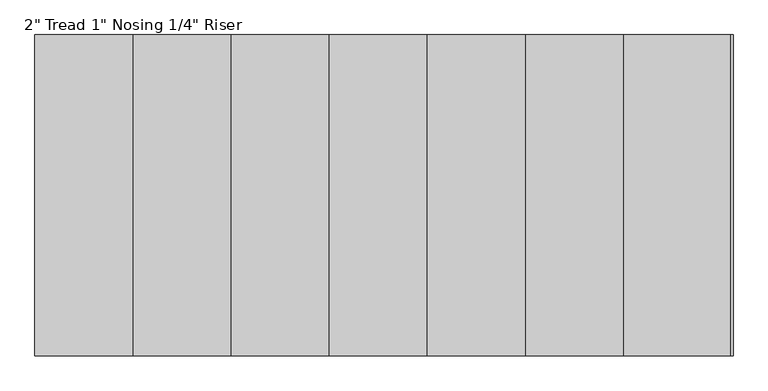
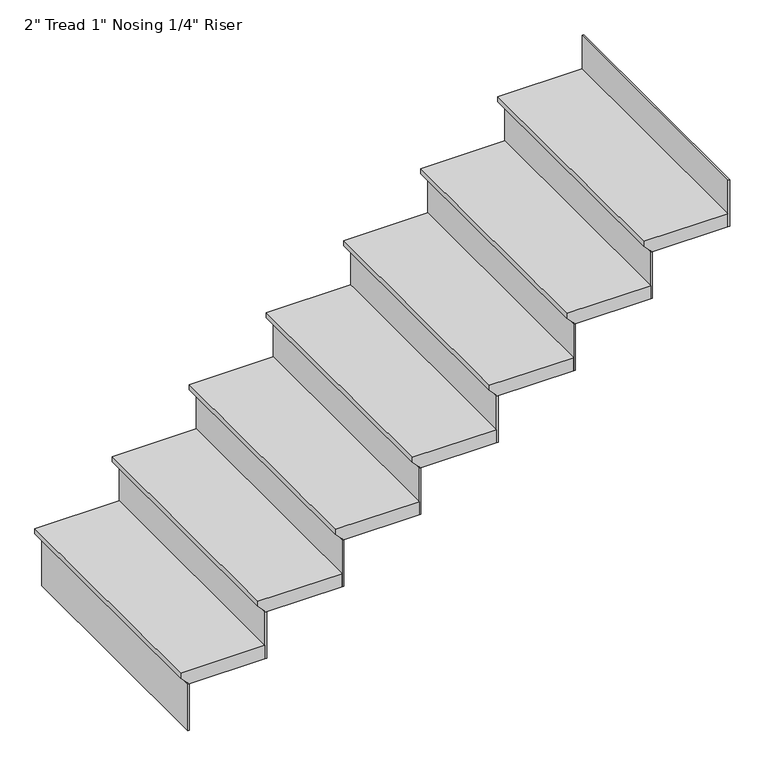
"""IFC4 building model written with IfcOpenShell, lengths in millimetres: stair flight geometry."""

from ifc_helpers import new_model, si_unit, frame, origin, place, context, project, spatial, polyline, outline, extrude, source, transform, mapped, element, save


def stair_flight_cba1433b(model_context):
    return source(origin(), model_context, "Body", "SweptSolid", [
        extrude(outline(polyline([(5765.8, -11753.6120641), (5765.8, -12058.4120641), (5746.75, -12058.4120641), (5721.35, -12033.0120641), (5715.0, -12033.0120641), (5715.0, -11753.6120641), (5765.8, -11753.6120641)])), frame((0.0, -4817.9038196, 0.0), z_axis=(0.0, 1.0, 0.0), x_axis=(0.0, 0.0, 1.0)), (0.0, 0.0, 1.0), 914.4),
        extrude(outline(polyline([(-12026.6620641, -4817.9038196), (-12033.0120641, -4817.9038196), (-12033.0120641, -3903.5038196), (-12026.6620641, -3903.5038196), (-12026.6620641, -4817.9038196)])), frame((0.0, 0.0, 5537.2), z_axis=(0.0, 0.0, 1.0), x_axis=(1.0, 0.0, 0.0)), (0.0, 0.0, 1.0), 177.8),
        extrude(outline(polyline([(-11747.2620641, -4817.9038196), (-11753.6120641, -4817.9038196), (-11753.6120641, -3903.5038196), (-11747.2620641, -3903.5038196), (-11747.2620641, -4817.9038196)])), frame((0.0, 0.0, 5715.0), z_axis=(0.0, 0.0, 1.0), x_axis=(1.0, 0.0, 0.0)), (0.0, 0.0, 1.0), 177.8),
        extrude(outline(polyline([(5943.6, -11474.2120641), (5943.6, -11779.0120641), (5924.55, -11779.0120641), (5899.15, -11753.6120641), (5892.8, -11753.6120641), (5892.8, -11474.2120641), (5943.6, -11474.2120641)])), frame((0.0, -4817.9038196, 0.0), z_axis=(0.0, 1.0, 0.0), x_axis=(0.0, 0.0, 1.0)), (0.0, 0.0, 1.0), 914.4),
        extrude(outline(polyline([(-11467.8620641, -4817.9038196), (-11474.2120641, -4817.9038196), (-11474.2120641, -3903.5038196), (-11467.8620641, -3903.5038196), (-11467.8620641, -4817.9038196)])), frame((0.0, 0.0, 5892.8), z_axis=(0.0, 0.0, 1.0), x_axis=(1.0, 0.0, 0.0)), (0.0, 0.0, 1.0), 177.8),
        extrude(outline(polyline([(6121.4, -11194.8120641), (6121.4, -11499.6120641), (6102.35, -11499.6120641), (6076.95, -11474.2120641), (6070.6, -11474.2120641), (6070.6, -11194.8120641), (6121.4, -11194.8120641)])), frame((0.0, -4817.9038196, 0.0), z_axis=(0.0, 1.0, 0.0), x_axis=(0.0, 0.0, 1.0)), (0.0, 0.0, 1.0), 914.4),
        extrude(outline(polyline([(-11188.4620641, -4817.9038196), (-11194.8120641, -4817.9038196), (-11194.8120641, -3903.5038196), (-11188.4620641, -3903.5038196), (-11188.4620641, -4817.9038196)])), frame((0.0, 0.0, 6070.6), z_axis=(0.0, 0.0, 1.0), x_axis=(1.0, 0.0, 0.0)), (0.0, 0.0, 1.0), 177.8),
        extrude(outline(polyline([(6299.2, -10915.4120641), (6299.2, -11220.2120641), (6280.15, -11220.2120641), (6254.75, -11194.8120641), (6248.4, -11194.8120641), (6248.4, -10915.4120641), (6299.2, -10915.4120641)])), frame((0.0, -4817.9038196, 0.0), z_axis=(0.0, 1.0, 0.0), x_axis=(0.0, 0.0, 1.0)), (0.0, 0.0, 1.0), 914.4),
        extrude(outline(polyline([(-10909.0620641, -4817.9038196), (-10915.4120641, -4817.9038196), (-10915.4120641, -3903.5038196), (-10909.0620641, -3903.5038196), (-10909.0620641, -4817.9038196)])), frame((0.0, 0.0, 6248.4), z_axis=(0.0, 0.0, 1.0), x_axis=(1.0, 0.0, 0.0)), (0.0, 0.0, 1.0), 177.8),
        extrude(outline(polyline([(6477.0, -10636.0120641), (6477.0, -10940.8120641), (6457.95, -10940.8120641), (6432.55, -10915.4120641), (6426.2, -10915.4120641), (6426.2, -10636.0120641), (6477.0, -10636.0120641)])), frame((0.0, -4817.9038196, 0.0), z_axis=(0.0, 1.0, 0.0), x_axis=(0.0, 0.0, 1.0)), (0.0, 0.0, 1.0), 914.4),
        extrude(outline(polyline([(-10629.6620641, -4817.9038196), (-10636.0120641, -4817.9038196), (-10636.0120641, -3903.5038196), (-10629.6620641, -3903.5038196), (-10629.6620641, -4817.9038196)])), frame((0.0, 0.0, 6426.2), z_axis=(0.0, 0.0, 1.0), x_axis=(1.0, 0.0, 0.0)), (0.0, 0.0, 1.0), 177.8),
        extrude(outline(polyline([(6654.8, -10356.6120641), (6654.8, -10661.4120641), (6635.75, -10661.4120641), (6610.35, -10636.0120641), (6604.0, -10636.0120641), (6604.0, -10356.6120641), (6654.8, -10356.6120641)])), frame((0.0, -4817.9038196, 0.0), z_axis=(0.0, 1.0, 0.0), x_axis=(0.0, 0.0, 1.0)), (0.0, 0.0, 1.0), 914.4),
        extrude(outline(polyline([(-10350.2620641, -4817.9038196), (-10356.6120641, -4817.9038196), (-10356.6120641, -3903.5038196), (-10350.2620641, -3903.5038196), (-10350.2620641, -4817.9038196)])), frame((0.0, 0.0, 6604.0), z_axis=(0.0, 0.0, 1.0), x_axis=(1.0, 0.0, 0.0)), (0.0, 0.0, 1.0), 177.8),
        extrude(outline(polyline([(-10070.8620641, -4817.9038196), (-10077.2120641, -4817.9038196), (-10077.2120641, -3903.5038196), (-10070.8620641, -3903.5038196), (-10070.8620641, -4817.9038196)])), frame((0.0, 0.0, 6781.8), z_axis=(0.0, 0.0, 1.0), x_axis=(1.0, 0.0, 0.0)), (0.0, 0.0, 1.0), 177.8),
        extrude(outline(polyline([(6832.6, -10077.2120641), (6832.6, -10382.0120641), (6813.55, -10382.0120641), (6788.15, -10356.6120641), (6781.8, -10356.6120641), (6781.8, -10077.2120641), (6832.6, -10077.2120641)])), frame((0.0, -4817.9038196, 0.0), z_axis=(0.0, 1.0, 0.0), x_axis=(0.0, 0.0, 1.0)), (0.0, 0.0, 1.0), 914.4),
    ])


if __name__ == "__main__":
    model = new_model("IFC4")
    model_context = context("Model", 3, world=origin())
    ifc_project = project(units=[si_unit("LENGTHUNIT", "METRE", prefix="MILLI")], contexts=[model_context])
    site = spatial("IfcSite", under=ifc_project)
    building = spatial("IfcBuilding", under=site)
    placement = place(None, origin())
    stair_flight_shape = stair_flight_cba1433b(model_context)
    element("IfcStairFlight", 1, ObjectType="2\" Tread 1\" Nosing 1/4\" Riser", at=placement, inside=building, context=model_context, shape_type="MappedRepresentation", body=[
        mapped(stair_flight_shape, transform((0.0, 0.0, 0.0), x_axis=(1.0, 0.0, 0.0), y_axis=(0.0, 1.0, 0.0), z_axis=(0.0, 0.0, 1.0))),
    ])
    save(model, "model.ifc")
